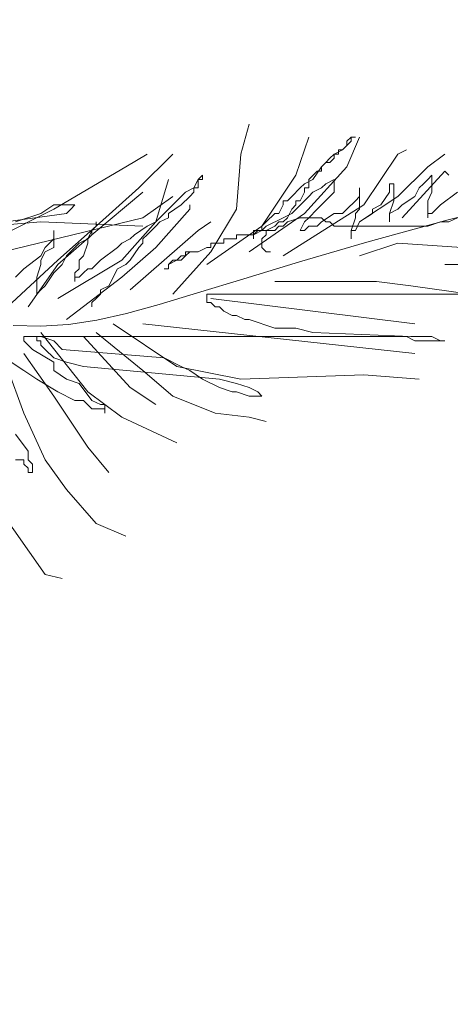
# Model space of a CAD drawing. Units: millimetres. Extents: x 595116 to 630915, y 909473 to 920225.
# Tile 25 of 134: x 629610.314 to 629613.214, y 919164.942 to 919171.576. Entities that reach past the tile are written whole.
import ezdxf

# ---------------------------------------------------------------- set-up
doc = ezdxf.new("R2010")
doc.units = ezdxf.units.MM
doc.layers.add('Dimension', color=3, linetype='Continuous', lineweight=18)
doc.layers.add('L-PLNT', color=85, linetype='Continuous', lineweight=13)
doc.styles.get("Standard").update_dxf_attribs({"font": 'arial.ttf'})
doc.dimstyles.new('ISO-25', dxfattribs={"dimtxt": 9, "dimasz": 6, "dimexe": 1.25, "dimexo": 0.625, "dimtad": 1, "dimlunit": 4, "dimtxsty": 'Standard', "dimcen": 2.5, "dimadec": 0, "dimazin": 0, "dimtfac": 1, "dimtmove": 0, "dimatfit": 3, "dimfxl": 1, "dimarcsym": 0})

# ---------------------------------------------------------------- blocks, each defined once
blk = doc.blocks.new('A$C4FB75ABC')
for p, q in [((4.2249, 2.058), (4.2402, 2.1114)), ((4.324, 2.0199), (4.3469, 2.0885)), ((4.4156, 2.0809), (4.4232, 2.0885)), ((4.4156, 2.0352), (4.4384, 2.0885)), ((4.4232, 2.0885), (4.4308, 2.0885)), ((4.4308, 2.0885), (4.4232, 2.0885)), ((4.4232, 2.0885), (4.4232, 2.0809)), ((4.4079, 2.0657), (4.4156, 2.0733)), ((4.4156, 2.0733), (4.4079, 2.0657)), ((4.4156, 2.0733), (4.4156, 2.0809)), ((4.4232, 2.0809), (4.4156, 2.0733)), ((4.019, 2.0352), (4.0571, 2.058)), ((4.0419, 1.9971), (4.1029, 2.058)), ((4.2173, 1.9589), (4.2249, 2.058)), ((4.3851, 2.0504), (4.3774, 2.0428)), ((4.3927, 2.058), (4.3851, 2.0504)), ((4.3851, 2.0428), (4.3927, 2.0504)), ((4.4079, 2.0657), (4.3927, 2.058)), ((4.3927, 2.0504), (4.3927, 2.058)), ((4.3927, 2.058), (4.4003, 2.058)), ((4.4003, 2.058), (4.4003, 2.0657)), ((4.4003, 2.0657), (4.4079, 2.0657)), ((4.4461, 1.9666), (4.5071, 2.058)), ((4.5071, 2.058), (4.5223, 2.0657)), ((4.5605, 2.0352), (4.591, 2.058)), ((3.8894, 1.9589), (4.019, 2.0352)), ((4.3393, 1.9513), (4.4156, 2.0352)), ((4.3698, 2.0352), (4.3546, 2.0123)), ((4.3698, 2.0352), (4.3774, 2.0428)), ((4.3774, 2.0428), (4.3698, 2.0352)), ((4.3698, 2.0275), (4.3698, 2.0352)), ((4.3774, 2.0428), (4.3851, 2.0428)), ((4.5071, 1.9818), (4.5605, 2.0352)), ((4.1563, 2.0199), (4.1486, 2.0123)), ((4.1563, 2.0123), (4.1563, 2.0199)), ((4.263, 1.9285), (4.324, 2.0199)), ((4.3469, 2.0123), (4.3622, 2.0275)), ((4.3622, 2.0275), (4.3698, 2.0275)), ((4.5147, 1.9437), (4.591, 2.0275)), ((4.5605, 2.0123), (4.5681, 2.0199)), ((4.5681, 2.0199), (4.5681, 1.9894)), ((4.591, 2.0275), (4.5986, 2.0199)), ((4.0724, 1.9361), (4.0953, 2.0123)), ((4.1486, 2.0123), (4.141, 1.9971)), ((4.1486, 1.9971), (4.1486, 2.0123)), ((4.1486, 2.0123), (4.1563, 2.0123)), ((4.3393, 2.0047), (4.3317, 1.9971)), ((4.3546, 2.0123), (4.3393, 2.0047)), ((4.3469, 1.9971), (4.3469, 2.0123)), ((4.3698, 1.9971), (4.3774, 2.0047)), ((4.3774, 2.0047), (4.3927, 2.0123)), ((4.3927, 2.0123), (4.3927, 1.9894)), ((4.4918, 1.9894), (4.4918, 2.0047)), ((4.4918, 2.0047), (4.4995, 2.0047)), ((4.4995, 2.0047), (4.4995, 1.9742)), ((4.5452, 1.9971), (4.5528, 2.0047)), ((4.5528, 2.0047), (4.5605, 2.0123)), ((3.958, 1.9132), (4.0495, 1.9894)), ((3.9656, 1.9285), (4.0419, 1.9971)), ((4.0495, 1.9437), (4.1029, 1.9818)), ((4.1181, 1.9818), (4.1029, 1.9666)), ((4.1258, 1.9894), (4.1181, 1.9818)), ((4.1181, 1.9666), (4.1334, 1.9818)), ((4.141, 1.9971), (4.1258, 1.9894)), ((4.1334, 1.9818), (4.141, 1.9894)), ((4.141, 1.9894), (4.141, 1.9971)), ((4.141, 1.9971), (4.1486, 1.9971)), ((4.3164, 1.9818), (4.3088, 1.9742)), ((4.3317, 1.9971), (4.3164, 1.9818)), ((4.3164, 1.9513), (4.3469, 1.9818)), ((4.3317, 1.9742), (4.3393, 1.9894)), ((4.3393, 1.9894), (4.3393, 1.9971)), ((4.3393, 1.9971), (4.3469, 1.9971)), ((4.3469, 1.9818), (4.3546, 1.9894)), ((4.3546, 1.9894), (4.3698, 1.9971)), ((4.3851, 1.9818), (4.3698, 1.9666)), ((4.3927, 1.9894), (4.3851, 1.9818)), ((4.4308, 1.9742), (4.4384, 1.9818)), ((4.4384, 1.9818), (4.4384, 1.9971)), ((4.4384, 1.9971), (4.4384, 1.9589)), ((4.4384, 1.9361), (4.5071, 1.9818)), ((4.4766, 1.9666), (4.4918, 1.9894)), ((4.5147, 1.9666), (4.5376, 1.9818)), ((4.5376, 1.9818), (4.5452, 1.9971)), ((4.5681, 1.9894), (4.5605, 1.9742)), ((4.5833, 1.9666), (4.6138, 1.9894)), ((4.7725, 1.9851), (4.5975, 1.9398)), ((3.8894, 1.9666), (3.8665, 1.9513)), ((3.9275, 1.9666), (3.8894, 1.9666)), ((3.9199, 1.9589), (3.9275, 1.9666)), ((4.1029, 1.9666), (4.08, 1.9437)), ((4.0953, 1.9513), (4.1181, 1.9666)), ((4.1334, 1.9589), (4.1334, 1.9666)), ((4.3012, 1.9666), (4.2935, 1.9513)), ((4.3088, 1.9742), (4.3012, 1.9742)), ((4.3012, 1.9742), (4.3012, 1.9666)), ((4.3012, 1.8751), (4.4461, 1.9666)), ((4.3164, 1.9589), (4.324, 1.9666)), ((4.324, 1.9666), (4.324, 1.9742)), ((4.324, 1.9742), (4.3317, 1.9742)), ((4.3698, 1.9666), (4.3622, 1.9589)), ((4.4156, 1.9589), (4.4308, 1.9742)), ((4.4613, 1.9589), (4.4766, 1.9666)), ((4.4995, 1.9742), (4.4918, 1.9513)), ((4.5071, 1.9589), (4.5147, 1.9666)), ((4.5605, 1.9742), (4.5605, 1.9437)), ((4.5757, 1.9589), (4.5833, 1.9666)), ((3.7445, 1.9285), (3.9122, 1.9513)), ((3.7521, 1.8903), (3.8894, 1.9589)), ((3.8665, 1.9513), (3.8207, 1.9361)), ((3.9122, 1.9513), (3.9199, 1.9589)), ((4.0724, 1.8903), (4.1334, 1.9589)), ((4.0953, 1.9437), (4.0953, 1.9513)), ((4.1715, 1.8827), (4.2173, 1.9589)), ((4.2402, 1.8827), (4.3393, 1.9513)), ((4.2859, 1.9513), (4.2707, 1.9361)), ((4.2935, 1.9513), (4.2859, 1.9513)), ((4.3012, 1.9437), (4.3164, 1.9513)), ((4.3088, 1.9437), (4.3164, 1.9589)), ((4.3622, 1.9589), (4.3469, 1.9437)), ((4.3698, 1.9361), (4.3927, 1.9513)), ((4.3927, 1.9513), (4.4079, 1.9513)), ((4.4079, 1.9513), (4.4156, 1.9589)), ((4.4384, 1.9589), (4.4308, 1.9513)), ((4.4308, 1.9513), (4.4308, 1.9437)), ((4.4384, 1.9361), (4.4613, 1.9513)), ((4.4613, 1.9513), (4.4613, 1.9589)), ((4.4918, 1.9513), (4.5071, 1.9589)), ((4.4918, 1.9513), (4.4918, 1.9361)), ((4.4918, 1.9361), (4.4918, 1.9513)), ((4.5605, 1.9513), (4.5681, 1.9513)), ((4.5605, 1.9437), (4.5605, 1.9513)), ((4.5681, 1.9513), (4.5757, 1.9589)), ((3.5843, 1.9132), (3.8665, 1.9361)), ((3.7978, 1.8827), (4.0495, 1.9437)), ((3.8665, 1.9361), (4.0495, 1.9285)), ((3.897, 1.8675), (3.9656, 1.9285)), ((3.958, 1.9208), (3.9656, 1.9285)), ((3.9656, 1.9285), (3.958, 1.9208)), ((3.9656, 1.9285), (3.9656, 1.9361)), ((3.9656, 1.9361), (3.9656, 1.9285)), ((4.0114, 1.8675), (4.0724, 1.9361)), ((4.0571, 1.9285), (4.0343, 1.9132)), ((4.0724, 1.9361), (4.0571, 1.9285)), ((4.0571, 1.9132), (4.0724, 1.9285)), ((4.08, 1.9437), (4.0724, 1.9361)), ((4.0724, 1.9285), (4.08, 1.9361)), ((4.08, 1.9361), (4.0953, 1.9437)), ((4.1486, 1.9208), (4.1715, 1.9361)), ((4.1639, 1.8599), (4.263, 1.9285)), ((4.2707, 1.9361), (4.263, 1.9285)), ((4.263, 1.9285), (4.263, 1.9208)), ((4.263, 1.9208), (4.2707, 1.9285)), ((4.2707, 1.9285), (4.3012, 1.9437)), ((4.2707, 1.9208), (4.2859, 1.9285)), ((4.2859, 1.9285), (4.2935, 1.9361)), ((4.2935, 1.9285), (4.2859, 1.9208)), ((4.2935, 1.9361), (4.3012, 1.9361)), ((4.3012, 1.9285), (4.2935, 1.9285)), ((4.3012, 1.9361), (4.3088, 1.9437)), ((4.3088, 1.9361), (4.3012, 1.9285)), ((4.3317, 1.9437), (4.3088, 1.9361)), ((4.3698, 1.9437), (4.3317, 1.9437)), ((4.3393, 1.9361), (4.3317, 1.9208)), ((4.3469, 1.9437), (4.3393, 1.9361)), ((4.3393, 1.9208), (4.3469, 1.9285)), ((4.3469, 1.9285), (4.3622, 1.9285)), ((4.3622, 1.9285), (4.3698, 1.9361)), ((4.3774, 1.9361), (4.3698, 1.9437)), ((4.3851, 1.9361), (4.3774, 1.9361)), ((4.3927, 1.9285), (4.3851, 1.9361)), ((4.5605, 1.9285), (4.3927, 1.9285)), ((4.4308, 1.9437), (4.4232, 1.9208)), ((4.4308, 1.9208), (4.4384, 1.9361)), ((4.5975, 1.9398), (4.4513, 1.8996)), ((4.5833, 1.9361), (4.5605, 1.9285)), ((4.5986, 1.9361), (4.5833, 1.9361)), ((4.6138, 1.9437), (4.5986, 1.9361)), ((3.8894, 1.8903), (3.8894, 1.9208)), ((3.8894, 1.9208), (3.8894, 1.9056)), ((3.897, 1.8599), (3.958, 1.9132)), ((3.958, 1.9208), (3.9504, 1.9056)), ((3.9504, 1.9056), (3.958, 1.9132)), ((3.958, 1.9132), (3.958, 1.9208)), ((4.0266, 1.8141), (4.1486, 1.9208)), ((4.0343, 1.9132), (4.0266, 1.9056)), ((4.0495, 1.9056), (4.0571, 1.9132)), ((4.2478, 1.9132), (4.2173, 1.9132)), ((4.2173, 1.9132), (4.2173, 1.9056)), ((4.2554, 1.9208), (4.2478, 1.9132)), ((4.2478, 1.9056), (4.2478, 1.9208)), ((4.2478, 1.9208), (4.263, 1.9208)), ((4.263, 1.9208), (4.2478, 1.9132)), ((4.2478, 1.9132), (4.2478, 1.9056)), ((4.263, 1.9208), (4.2554, 1.9208)), ((4.2859, 1.9208), (4.263, 1.9208)), ((4.263, 1.9056), (4.2707, 1.9132)), ((4.2707, 1.9132), (4.2707, 1.9208)), ((4.3317, 1.9208), (4.3393, 1.9208)), ((4.4232, 1.9208), (4.4232, 1.9056)), ((4.4232, 1.9056), (4.4232, 1.9208)), ((4.4232, 1.9208), (4.4308, 1.9208)), ((3.8894, 1.9056), (3.8741, 1.8903)), ((3.9351, 1.898), (3.9122, 1.8751)), ((3.9504, 1.9056), (3.9351, 1.898)), ((3.9427, 1.8751), (3.9504, 1.898)), ((3.9504, 1.898), (3.9504, 1.9056)), ((4.0114, 1.898), (4.0037, 1.8903)), ((4.0266, 1.9056), (4.0114, 1.898)), ((4.0419, 1.8903), (4.0495, 1.898)), ((4.0495, 1.898), (4.0495, 1.9056)), ((4.1944, 1.898), (4.1715, 1.898)), ((4.1715, 1.898), (4.1715, 1.8903)), ((4.2173, 1.9056), (4.1944, 1.9056)), ((4.1944, 1.9056), (4.1944, 1.898)), ((4.263, 1.8903), (4.263, 1.9056)), ((4.4513, 1.8996), (4.3302, 1.8644)), ((4.4384, 1.8751), (4.5071, 1.898)), ((4.5071, 1.898), (4.6215, 1.8903)), ((3.8665, 1.8751), (3.836, 1.8522)), ((3.8741, 1.8903), (3.8665, 1.8751)), ((3.8665, 1.8675), (3.8741, 1.8827)), ((3.8741, 1.8827), (3.8894, 1.8903)), ((3.9122, 1.8751), (3.9046, 1.8599)), ((3.9351, 1.8675), (3.9427, 1.8751)), ((4.0037, 1.8903), (3.9732, 1.8675)), ((4.0114, 1.837), (4.0724, 1.8903)), ((4.0266, 1.8675), (4.0419, 1.8903)), ((4.1029, 1.8065), (4.1715, 1.8827)), ((4.1181, 1.8751), (4.1105, 1.8675)), ((4.1258, 1.8751), (4.1181, 1.8751)), ((4.1181, 1.8675), (4.1258, 1.8751)), ((4.1334, 1.8827), (4.1258, 1.8751)), ((4.1258, 1.8751), (4.1258, 1.8827)), ((4.1258, 1.8827), (4.1334, 1.8827)), ((4.1486, 1.8827), (4.1334, 1.8827)), ((4.1639, 1.8903), (4.1486, 1.8827)), ((4.1715, 1.8903), (4.1639, 1.8903)), ((4.2707, 1.8827), (4.263, 1.8903)), ((4.2783, 1.8827), (4.2707, 1.8827)), ((3.7978, 1.776), (3.897, 1.8675)), ((3.8436, 1.7836), (3.897, 1.8599)), ((3.8589, 1.837), (3.8665, 1.8599)), ((3.8665, 1.8599), (3.8665, 1.8675)), ((3.9046, 1.8599), (3.8894, 1.8446)), ((3.897, 1.7989), (4.0114, 1.8675)), ((3.9351, 1.8522), (3.9351, 1.8675)), ((3.9656, 1.8599), (3.958, 1.8522)), ((3.9732, 1.8675), (3.9656, 1.8599)), ((4.0037, 1.8522), (4.019, 1.8599)), ((4.019, 1.8599), (4.0266, 1.8675)), ((4.1029, 1.8675), (4.0953, 1.8599)), ((4.0953, 1.8599), (4.1105, 1.8675)), ((4.0953, 1.8599), (4.0953, 1.8522)), ((4.0953, 1.8522), (4.0953, 1.8599)), ((4.1105, 1.8675), (4.1029, 1.8675)), ((4.1105, 1.8675), (4.1181, 1.8675)), ((4.3302, 1.8644), (4.2303, 1.8341)), ((4.6062, 1.8599), (4.591, 1.8599)), ((4.591, 1.8599), (4.652, 1.8599)), ((3.836, 1.8522), (3.8207, 1.837)), ((3.8894, 1.8446), (3.8741, 1.8217)), ((3.9275, 1.8446), (3.9351, 1.8522)), ((3.9275, 1.8294), (3.9275, 1.8446)), ((3.9427, 1.8446), (3.9351, 1.837)), ((3.9504, 1.8522), (3.9427, 1.8446)), ((3.958, 1.8522), (3.9504, 1.8522)), ((3.9885, 1.8217), (4.0037, 1.8522)), ((4.0953, 1.8522), (4.0876, 1.8522)), ((4.0876, 1.8522), (4.0953, 1.8522)), ((3.8589, 1.8065), (3.8589, 1.837)), ((3.8741, 1.8217), (3.8665, 1.8141)), ((3.9122, 1.7608), (4.0114, 1.837)), ((3.9351, 1.837), (3.9275, 1.837)), ((3.9275, 1.837), (3.9275, 1.8294)), ((3.9732, 1.8141), (3.9885, 1.8217)), ((4.2303, 1.8341), (4.1477, 1.8087)), ((4.2859, 1.8294), (4.4689, 1.8294)), ((4.4689, 1.8294), (4.53, 1.8217)), ((4.53, 1.8217), (4.6367, 1.8065)), ((3.8665, 1.8141), (3.8589, 1.8065)), ((3.9656, 1.7989), (3.9732, 1.8065)), ((3.9732, 1.8065), (3.9732, 1.8141)), ((4.1477, 1.8087), (4.0788, 1.7878)), ((4.1639, 1.7913), (4.1639, 1.8065)), ((4.1639, 1.8065), (5.0333, 1.8065)), ((3.958, 1.7913), (3.9656, 1.7989)), ((3.958, 1.7836), (3.958, 1.7913)), ((4.0788, 1.7878), (4.0197, 1.7715)), ((4.1715, 1.7913), (4.1639, 1.7913)), ((4.1715, 1.7989), (4.5376, 1.7531)), ((4.1792, 1.7836), (4.1715, 1.7913)), ((4.0197, 1.7715), (3.9666, 1.7597)), ((4.1868, 1.7836), (4.1792, 1.7836)), ((4.1944, 1.776), (4.1868, 1.7836)), ((4.2097, 1.7684), (4.1944, 1.776)), ((4.2173, 1.7684), (4.2097, 1.7684)), ((4.2325, 1.7608), (4.2173, 1.7684)), ((3.8664, 1.749), (3.8165, 1.7504)), ((3.916, 1.7521), (3.8664, 1.749)), ((3.9666, 1.7597), (3.916, 1.7521)), ((3.9961, 1.7531), (4.1105, 1.6769)), ((4.0495, 1.7531), (4.5376, 1.6998)), ((4.2402, 1.7608), (4.2325, 1.7608)), ((4.2859, 1.7455), (4.2402, 1.7608)), ((3.8665, 1.7379), (3.9504, 1.6312)), ((3.9656, 1.7379), (4.0495, 1.6693)), ((4.324, 1.7455), (4.2859, 1.7455)), ((4.3546, 1.7379), (4.324, 1.7455)), ((4.53, 1.7303), (4.3546, 1.7379)), ((3.836, 1.7227), (3.836, 1.7303)), ((3.836, 1.7303), (3.8665, 1.7303)), ((3.8436, 1.715), (3.836, 1.7227)), ((3.8512, 1.7074), (3.8436, 1.715)), ((3.8589, 1.7227), (3.8589, 1.7303)), ((3.8589, 1.7303), (4.5223, 1.7303)), ((3.8665, 1.7227), (3.8589, 1.7227)), ((3.8665, 1.7303), (3.8894, 1.7227)), ((3.8665, 1.715), (3.8665, 1.7227)), ((3.8741, 1.7074), (3.8665, 1.715)), ((3.8894, 1.7227), (3.9046, 1.7074)), ((3.9427, 1.7303), (4.0266, 1.6388)), ((4.5223, 1.7303), (4.5376, 1.7227)), ((4.5681, 1.7303), (4.53, 1.7303)), ((4.5376, 1.7227), (4.591, 1.7227)), ((4.5833, 1.7227), (4.5681, 1.7303)), ((4.591, 1.7227), (4.5833, 1.7227)), ((3.836, 1.6998), (3.8894, 1.6236)), ((3.8894, 1.6845), (3.8512, 1.7074)), ((3.8894, 1.6922), (3.8741, 1.7074)), ((3.9046, 1.7074), (4.0876, 1.6922)), ((3.8131, 1.6845), (3.836, 1.6693)), ((3.9122, 1.6845), (3.8894, 1.6922)), ((3.8894, 1.6693), (3.8894, 1.6845)), ((3.9427, 1.6769), (3.9122, 1.6845)), ((4.0876, 1.6922), (4.1181, 1.6769)), ((3.8055, 1.6769), (3.836, 1.5931)), ((3.836, 1.6693), (3.8589, 1.6541)), ((3.9122, 1.6541), (3.8894, 1.6693)), ((4.1868, 1.6541), (3.9427, 1.6769)), ((4.0495, 1.6693), (4.1029, 1.6236)), ((4.1105, 1.6769), (4.2249, 1.6541)), ((4.1181, 1.6769), (4.1334, 1.6693)), ((4.1334, 1.6693), (4.1563, 1.6541)), ((4.2249, 1.6541), (4.4461, 1.6617)), ((4.4461, 1.6617), (4.5452, 1.6541)), ((3.8589, 1.6541), (3.897, 1.6312)), ((3.9351, 1.6464), (3.9122, 1.6541)), ((3.958, 1.6159), (3.9351, 1.6464)), ((4.1563, 1.6541), (4.1868, 1.6388)), ((4.2173, 1.6464), (4.1868, 1.6541)), ((4.2402, 1.6388), (4.2173, 1.6464)), ((3.897, 1.6312), (3.9275, 1.6159)), ((3.9504, 1.6312), (4.0114, 1.5855)), ((4.0266, 1.6388), (4.0724, 1.6083)), ((4.1868, 1.6388), (4.2097, 1.6312)), ((4.2097, 1.6312), (4.2173, 1.6312)), ((4.2173, 1.6312), (4.2402, 1.6236)), ((4.2554, 1.6312), (4.2402, 1.6388)), ((4.263, 1.6236), (4.2554, 1.6312)), ((3.8894, 1.6236), (3.9504, 1.5321)), ((3.9275, 1.6159), (3.9427, 1.6159)), ((3.9427, 1.6159), (3.958, 1.6007)), ((3.9732, 1.6083), (3.958, 1.6159)), ((4.1029, 1.6236), (4.1792, 1.5931)), ((4.2402, 1.6236), (4.263, 1.6236)), ((3.836, 1.5931), (3.8741, 1.5092)), ((3.958, 1.6007), (3.9809, 1.6007)), ((3.9809, 1.6083), (3.9732, 1.6083)), ((3.9809, 1.5931), (3.9809, 1.6083)), ((3.9809, 1.6007), (3.9809, 1.5931)), ((4.1792, 1.5931), (4.2402, 1.5855)), ((4.0114, 1.5855), (4.1105, 1.5397)), ((4.2402, 1.5855), (4.2707, 1.5778)), ((3.8436, 1.5245), (3.8207, 1.555)), ((3.8436, 1.5092), (3.8436, 1.5245)), ((3.9504, 1.5321), (3.9885, 1.4864)), ((3.8207, 1.5092), (3.836, 1.5092)), ((3.836, 1.5092), (3.836, 1.5016)), ((3.8512, 1.5016), (3.8436, 1.5092)), ((3.8741, 1.5092), (3.9122, 1.4559)), ((3.836, 1.5016), (3.8436, 1.494)), ((3.8436, 1.494), (3.8436, 1.4864)), ((3.8436, 1.4864), (3.8512, 1.4864)), ((3.8512, 1.4864), (3.8512, 1.5016)), ((3.9122, 1.4559), (3.9656, 1.3949)), ((3.7826, 1.433), (3.8741, 1.3034)), ((3.9656, 1.3949), (4.019, 1.372)), ((3.8741, 1.3034), (3.9046, 1.2958))]:
    blk.add_line(p, q)
blk = doc.blocks.new('*D216')
at = {"layer": 'Defpoints', "color": 0, "transparency": 16777216}
for p in [(629743.5408, 919411.9276), (629505.0408, 919411.8279), (629743.5408, 918832.3776)]:
    blk.add_point(p, dxfattribs=at)
at = {"layer": 'Dimension', "color": 0, "lineweight": -2, "transparency": 16777216}
for p, q in [((629743.5408, 919411.3026), (629743.5408, 918831.1276)), ((629505.0408, 919411.2029), (629505.0408, 918831.1276)), ((629511.0408, 918832.3776), (629737.5408, 918832.3776))]:
    blk.add_line(p, q, dxfattribs=at)
at = {"layer": 'Dimension', "color": 0, "transparency": 16777216}
for points in [[(629511.0408, 918833.3776), (629511.0408, 918831.3776), (629505.0408, 918832.3776)], [(629737.5408, 918833.3776), (629737.5408, 918831.3776), (629743.5408, 918832.3776)]]:
    blk.add_solid(points, dxfattribs=at)
at = {"layer": 'Dimension', "color": 0, "transparency": 16777216, "insert": (629624.2908, 918837.656), "char_height": 9, "attachment_point": 5}
blk.add_mtext('19\'-10 1/2"', dxfattribs=at)

msp = doc.modelspace()

# ---------------------------------------------------------------- block references
at = {"layer": 'L-PLNT', "xscale": 3.753413438031968, "yscale": 3.753413438031968, "zscale": 3.753413438031968}
msp.add_blockref('A$C4FB75ABC', (629595.9442, 919162.9458), dxfattribs=at)

# ---------------------------------------------------------------- dimensions: what is measured, and where the dimension line sits
at = {"layer": 'Dimension'}
dim = msp.add_linear_dim(base=(629743.5408, 918832.3776), p1=(629505.0408, 919411.8279), p2=(629743.5408, 919411.9276), dimstyle='ISO-25', override={"dimdec": 1, "dimlfac": 1, "dimrnd": 0, "dimzin": 1, "dimdsep": 46, "dimlunit": 4, "dimfrac": 2}, dxfattribs=at)
dim.commit()
dim.dimension.update_dxf_attribs({"geometry": '*D216', "text_midpoint": (629624.2908, 918837.656)})

doc.saveas('drawing.dxf')
